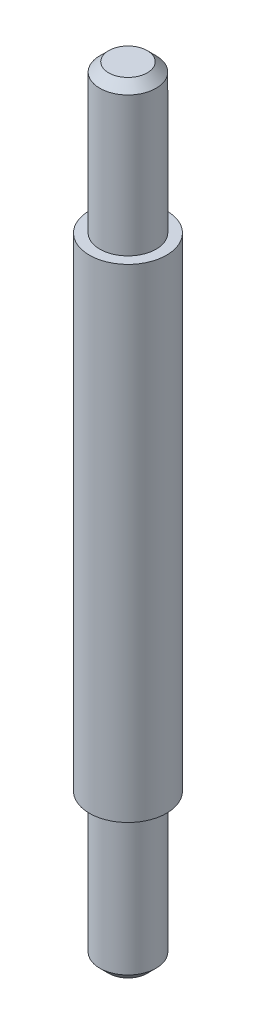
ISO-10303-21;
HEADER;
FILE_DESCRIPTION(('STEP AP214'),'2;1');
FILE_NAME('part.step','',(''),(''),'','','');
FILE_SCHEMA(('AUTOMOTIVE_DESIGN { 1 0 10303 214 1 1 1 1 }'));
ENDSEC;
DATA;
#1=APPLICATION_CONTEXT('core data for automotive mechanical design processes');
#2=APPLICATION_PROTOCOL_DEFINITION('international standard','automotive_design',2000,#1);
#3=PRODUCT_CONTEXT('',#1,'mechanical');
#4=PRODUCT('Part','Part','',(#3));
#5=PRODUCT_RELATED_PRODUCT_CATEGORY('part','',(#4));
#6=PRODUCT_DEFINITION_FORMATION('','',#4);
#7=PRODUCT_DEFINITION_CONTEXT('part definition',#1,'design');
#8=PRODUCT_DEFINITION('design','',#6,#7);
#9=PRODUCT_DEFINITION_SHAPE('','',#8);
#10=(LENGTH_UNIT() NAMED_UNIT(*) SI_UNIT(.MILLI.,.METRE.));
#11=(NAMED_UNIT(*) PLANE_ANGLE_UNIT() SI_UNIT($,.RADIAN.));
#12=(NAMED_UNIT(*) SI_UNIT($,.STERADIAN.) SOLID_ANGLE_UNIT());
#13=UNCERTAINTY_MEASURE_WITH_UNIT(LENGTH_MEASURE(1.E-05),#10,'distance_accuracy_value','');
#14=(GEOMETRIC_REPRESENTATION_CONTEXT(3) GLOBAL_UNCERTAINTY_ASSIGNED_CONTEXT((#13)) GLOBAL_UNIT_ASSIGNED_CONTEXT((#10,
#11,#12)) REPRESENTATION_CONTEXT('',''));
#15=CARTESIAN_POINT('',(0.,0.,0.));
#16=DIRECTION('',(0.,0.,1.));
#17=DIRECTION('',(1.,0.,0.));
#18=AXIS2_PLACEMENT_3D('',#15,#16,#17);
#19=CARTESIAN_POINT('',(0.,131.5,0.));
#20=DIRECTION('',(0.,-1.,0.));
#21=DIRECTION('',(0.,0.,-1.));
#22=AXIS2_PLACEMENT_3D('',#19,#20,#21);
#23=PLANE('',#22);
#24=CARTESIAN_POINT('',(0.,131.5,0.));
#25=DIRECTION('',(0.,-1.,0.));
#26=DIRECTION('',(0.,0.,-1.));
#27=AXIS2_PLACEMENT_3D('',#24,#25,#26);
#28=CIRCLE('',#27,6.50000000000003);
#29=CARTESIAN_POINT('',(0.,131.5,-6.50000000000003));
#30=VERTEX_POINT('',#29);
#31=EDGE_CURVE('E50',#30,#30,#28,.F.);
#32=ORIENTED_EDGE('',*,*,#31,.T.);
#33=EDGE_LOOP('',(#32));
#34=FACE_BOUND('',#33,.T.);
#35=ADVANCED_FACE('F39',(#34),#23,.F.);
#36=CARTESIAN_POINT('',(0.,65.5594059405942,0.));
#37=DIRECTION('',(0.,1.,0.));
#38=DIRECTION('',(0.,0.,1.));
#39=AXIS2_PLACEMENT_3D('',#36,#37,#38);
#40=CYLINDRICAL_SURFACE('',#39,9.49999999999999);
#41=CARTESIAN_POINT('',(0.,128.5,0.));
#42=DIRECTION('',(0.,-1.,0.));
#43=DIRECTION('',(0.,0.,-1.));
#44=AXIS2_PLACEMENT_3D('',#41,#42,#43);
#45=CIRCLE('',#44,9.49999999999999);
#46=CARTESIAN_POINT('',(0.,128.5,-9.49999999999999));
#47=VERTEX_POINT('',#46);
#48=EDGE_CURVE('E10',#47,#47,#45,.T.);
#49=ORIENTED_EDGE('',*,*,#48,.T.);
#50=EDGE_LOOP('',(#49));
#51=FACE_BOUND('',#50,.T.);
#52=CARTESIAN_POINT('',(0.,81.5,0.));
#53=DIRECTION('',(0.,1.,0.));
#54=DIRECTION('',(0.,0.,1.));
#55=AXIS2_PLACEMENT_3D('',#52,#53,#54);
#56=CIRCLE('',#55,9.49999999999999);
#57=CARTESIAN_POINT('',(0.,81.5,9.49999999999999));
#58=VERTEX_POINT('',#57);
#59=EDGE_CURVE('E58',#58,#58,#56,.T.);
#60=ORIENTED_EDGE('',*,*,#59,.T.);
#61=EDGE_LOOP('',(#60));
#62=FACE_BOUND('',#61,.T.);
#63=ADVANCED_FACE('F95',(#51,#62),#40,.T.);
#64=CARTESIAN_POINT('',(9.49999999999999,81.5,0.));
#65=DIRECTION('',(0.,-1.,0.));
#66=DIRECTION('',(0.,0.,-1.));
#67=AXIS2_PLACEMENT_3D('',#64,#65,#66);
#68=PLANE('',#67);
#69=ORIENTED_EDGE('',*,*,#59,.F.);
#70=EDGE_LOOP('',(#69));
#71=FACE_BOUND('',#70,.T.);
#72=CARTESIAN_POINT('',(0.,81.5,0.));
#73=DIRECTION('',(0.,1.,0.));
#74=DIRECTION('',(0.,0.,1.));
#75=AXIS2_PLACEMENT_3D('',#72,#73,#74);
#76=CIRCLE('',#75,13.);
#77=CARTESIAN_POINT('',(0.,81.5,13.));
#78=VERTEX_POINT('',#77);
#79=EDGE_CURVE('E64',#78,#78,#76,.T.);
#80=ORIENTED_EDGE('',*,*,#79,.T.);
#81=EDGE_LOOP('',(#80));
#82=FACE_BOUND('',#81,.T.);
#83=ADVANCED_FACE('F96',(#71,#82),#68,.F.);
#84=CARTESIAN_POINT('',(0.,65.5594059405942,0.));
#85=DIRECTION('',(0.,1.,0.));
#86=DIRECTION('',(0.,0.,1.));
#87=AXIS2_PLACEMENT_3D('',#84,#85,#86);
#88=CYLINDRICAL_SURFACE('',#87,13.);
#89=ORIENTED_EDGE('',*,*,#79,.F.);
#90=EDGE_LOOP('',(#89));
#91=FACE_BOUND('',#90,.T.);
#92=CARTESIAN_POINT('',(0.,-81.5,0.));
#93=DIRECTION('',(0.,1.,0.));
#94=DIRECTION('',(0.,0.,1.));
#95=AXIS2_PLACEMENT_3D('',#92,#93,#94);
#96=CIRCLE('',#95,13.0000000000001);
#97=CARTESIAN_POINT('',(0.,-81.5,13.0000000000001));
#98=VERTEX_POINT('',#97);
#99=EDGE_CURVE('E67',#98,#98,#96,.T.);
#100=ORIENTED_EDGE('',*,*,#99,.T.);
#101=EDGE_LOOP('',(#100));
#102=FACE_BOUND('',#101,.T.);
#103=ADVANCED_FACE('F86',(#91,#102),#88,.T.);
#104=CARTESIAN_POINT('',(13.0000000000001,-81.5,0.));
#105=DIRECTION('',(0.,1.,0.));
#106=DIRECTION('',(0.,0.,1.));
#107=AXIS2_PLACEMENT_3D('',#104,#105,#106);
#108=PLANE('',#107);
#109=ORIENTED_EDGE('',*,*,#99,.F.);
#110=EDGE_LOOP('',(#109));
#111=FACE_BOUND('',#110,.T.);
#112=CARTESIAN_POINT('',(0.,-81.5,0.));
#113=DIRECTION('',(0.,1.,0.));
#114=DIRECTION('',(0.,0.,1.));
#115=AXIS2_PLACEMENT_3D('',#112,#113,#114);
#116=CIRCLE('',#115,9.5);
#117=CARTESIAN_POINT('',(0.,-81.5,9.5));
#118=VERTEX_POINT('',#117);
#119=EDGE_CURVE('E69',#118,#118,#116,.T.);
#120=ORIENTED_EDGE('',*,*,#119,.T.);
#121=EDGE_LOOP('',(#120));
#122=FACE_BOUND('',#121,.T.);
#123=ADVANCED_FACE('F71',(#111,#122),#108,.F.);
#124=CARTESIAN_POINT('',(0.,65.5594059405942,0.));
#125=DIRECTION('',(0.,1.,0.));
#126=DIRECTION('',(0.,0.,1.));
#127=AXIS2_PLACEMENT_3D('',#124,#125,#126);
#128=CYLINDRICAL_SURFACE('',#127,9.50000000000001);
#129=CARTESIAN_POINT('',(0.,-128.5,0.));
#130=DIRECTION('',(0.,1.,0.));
#131=DIRECTION('',(0.,0.,1.));
#132=AXIS2_PLACEMENT_3D('',#129,#130,#131);
#133=CIRCLE('',#132,9.50000000000001);
#134=CARTESIAN_POINT('',(0.,-128.5,9.5));
#135=VERTEX_POINT('',#134);
#136=EDGE_CURVE('E54',#135,#135,#133,.T.);
#137=ORIENTED_EDGE('',*,*,#136,.T.);
#138=EDGE_LOOP('',(#137));
#139=FACE_BOUND('',#138,.T.);
#140=ORIENTED_EDGE('',*,*,#119,.F.);
#141=EDGE_LOOP('',(#140));
#142=FACE_BOUND('',#141,.T.);
#143=ADVANCED_FACE('F73',(#139,#142),#128,.T.);
#144=CARTESIAN_POINT('',(9.50000000000002,-131.5,0.));
#145=DIRECTION('',(0.,1.,0.));
#146=DIRECTION('',(0.,0.,1.));
#147=AXIS2_PLACEMENT_3D('',#144,#145,#146);
#148=PLANE('',#147);
#149=CARTESIAN_POINT('',(0.,-131.5,0.));
#150=DIRECTION('',(0.,1.,0.));
#151=DIRECTION('',(0.,0.,1.));
#152=AXIS2_PLACEMENT_3D('',#149,#150,#151);
#153=CIRCLE('',#152,6.50000000000003);
#154=CARTESIAN_POINT('',(0.,-131.5,6.50000000000002));
#155=VERTEX_POINT('',#154);
#156=EDGE_CURVE('E51',#155,#155,#153,.F.);
#157=ORIENTED_EDGE('',*,*,#156,.T.);
#158=EDGE_LOOP('',(#157));
#159=FACE_BOUND('',#158,.T.);
#160=ADVANCED_FACE('F80',(#159),#148,.F.);
#161=CARTESIAN_POINT('',(0.,-128.5,0.));
#162=DIRECTION('',(0.,1.,0.));
#163=DIRECTION('',(0.,0.,1.));
#164=AXIS2_PLACEMENT_3D('',#161,#162,#163);
#165=CONICAL_SURFACE('',#164,9.50000000000001,0.785398163397449);
#166=CARTESIAN_POINT('',(0.,-131.5,6.50000000000002));
#167=CARTESIAN_POINT('',(0.,-131.46875,6.53125000000002));
#168=CARTESIAN_POINT('',(0.,-131.4375,6.56250000000002));
#169=CARTESIAN_POINT('',(0.,-131.375,6.62500000000002));
#170=CARTESIAN_POINT('',(0.,-131.34375,6.65625000000002));
#171=CARTESIAN_POINT('',(0.,-131.28125,6.71875000000002));
#172=CARTESIAN_POINT('',(0.,-131.25,6.75000000000002));
#173=CARTESIAN_POINT('',(0.,-131.1875,6.81250000000002));
#174=CARTESIAN_POINT('',(0.,-131.15625,6.84375000000002));
#175=CARTESIAN_POINT('',(0.,-131.09375,6.90625000000002));
#176=CARTESIAN_POINT('',(0.,-131.0625,6.93750000000002));
#177=CARTESIAN_POINT('',(0.,-131.,7.00000000000001));
#178=CARTESIAN_POINT('',(0.,-130.96875,7.03125000000001));
#179=CARTESIAN_POINT('',(0.,-130.90625,7.09375000000001));
#180=CARTESIAN_POINT('',(0.,-130.875,7.12500000000002));
#181=CARTESIAN_POINT('',(0.,-130.8125,7.18750000000002));
#182=CARTESIAN_POINT('',(0.,-130.78125,7.21875000000001));
#183=CARTESIAN_POINT('',(0.,-130.71875,7.28125000000001));
#184=CARTESIAN_POINT('',(0.,-130.6875,7.31250000000001));
#185=CARTESIAN_POINT('',(0.,-130.625,7.37500000000001));
#186=CARTESIAN_POINT('',(0.,-130.59375,7.40625000000001));
#187=CARTESIAN_POINT('',(0.,-130.53125,7.46875000000001));
#188=CARTESIAN_POINT('',(0.,-130.5,7.50000000000001));
#189=CARTESIAN_POINT('',(0.,-130.4375,7.56250000000001));
#190=CARTESIAN_POINT('',(0.,-130.40625,7.59375000000001));
#191=CARTESIAN_POINT('',(0.,-130.34375,7.65625000000001));
#192=CARTESIAN_POINT('',(0.,-130.3125,7.68750000000001));
#193=CARTESIAN_POINT('',(0.,-130.25,7.75000000000001));
#194=CARTESIAN_POINT('',(0.,-130.21875,7.78125000000001));
#195=CARTESIAN_POINT('',(0.,-130.15625,7.84375000000001));
#196=CARTESIAN_POINT('',(0.,-130.125,7.87500000000001));
#197=CARTESIAN_POINT('',(0.,-130.0625,7.93750000000001));
#198=CARTESIAN_POINT('',(0.,-130.03125,7.96875000000001));
#199=CARTESIAN_POINT('',(0.,-129.96875,8.03125000000001));
#200=CARTESIAN_POINT('',(0.,-129.9375,8.06250000000001));
#201=CARTESIAN_POINT('',(0.,-129.875,8.12500000000001));
#202=CARTESIAN_POINT('',(0.,-129.84375,8.15625000000001));
#203=CARTESIAN_POINT('',(0.,-129.78125,8.21875000000001));
#204=CARTESIAN_POINT('',(0.,-129.75,8.25));
#205=CARTESIAN_POINT('',(0.,-129.6875,8.3125));
#206=CARTESIAN_POINT('',(0.,-129.65625,8.34375000000001));
#207=CARTESIAN_POINT('',(0.,-129.59375,8.40625000000001));
#208=CARTESIAN_POINT('',(0.,-129.5625,8.43750000000001));
#209=CARTESIAN_POINT('',(0.,-129.5,8.5));
#210=CARTESIAN_POINT('',(0.,-129.46875,8.53125));
#211=CARTESIAN_POINT('',(0.,-129.40625,8.59375));
#212=CARTESIAN_POINT('',(0.,-129.375,8.625));
#213=CARTESIAN_POINT('',(0.,-129.3125,8.6875));
#214=CARTESIAN_POINT('',(0.,-129.28125,8.71875));
#215=CARTESIAN_POINT('',(0.,-129.21875,8.78125));
#216=CARTESIAN_POINT('',(0.,-129.1875,8.8125));
#217=CARTESIAN_POINT('',(0.,-129.125,8.875));
#218=CARTESIAN_POINT('',(0.,-129.09375,8.90625));
#219=CARTESIAN_POINT('',(0.,-129.03125,8.96875000000001));
#220=CARTESIAN_POINT('',(0.,-129.,9.));
#221=CARTESIAN_POINT('',(0.,-128.9375,9.0625));
#222=CARTESIAN_POINT('',(0.,-128.90625,9.09375));
#223=CARTESIAN_POINT('',(0.,-128.84375,9.15625));
#224=CARTESIAN_POINT('',(0.,-128.8125,9.1875));
#225=CARTESIAN_POINT('',(0.,-128.75,9.25));
#226=CARTESIAN_POINT('',(0.,-128.71875,9.28125));
#227=CARTESIAN_POINT('',(0.,-128.65625,9.34375));
#228=CARTESIAN_POINT('',(0.,-128.625,9.375));
#229=CARTESIAN_POINT('',(0.,-128.5625,9.4375));
#230=CARTESIAN_POINT('',(0.,-128.53125,9.46875));
#231=CARTESIAN_POINT('',(0.,-128.5,9.5));
#232=B_SPLINE_CURVE_WITH_KNOTS('',3,(#166,#167,#168,#169,#170,#171,#172,#173,#174,#175,#176,
#177,#178,#179,#180,#181,#182,#183,#184,#185,#186,#187,#188,#189,#190,#191,#192,#193,#194,#195,
#196,#197,#198,#199,#200,#201,#202,#203,#204,#205,#206,#207,#208,#209,#210,#211,#212,#213,#214,
#215,#216,#217,#218,#219,#220,#221,#222,#223,#224,#225,#226,#227,#228,#229,#230,#231),
.UNSPECIFIED.,.F.,.F.,(4,2,2,2,2,2,2,2,2,2,2,2,2,2,2,2,2,2,2,2,2,2,2,2,2,2,2,2,2,2,2,2,4),(0.,
0.13258252147248,0.265165042944959,0.397747564417439,0.530330085889919,0.662912607362399,
0.795495128834879,0.928077650307338,1.06066017177982,1.1932426932523,1.32582521472478,
1.45840773619726,1.59099025766974,1.7235727791422,1.85615530061468,1.98873782208716,
2.12132034355964,2.25390286503212,2.3864853865046,2.51906790797708,2.65165042944954,
2.78423295092201,2.91681547239449,3.04939799386697,3.18198051533945,3.31456303681193,
3.44714555828439,3.57972807975687,3.71231060122935,3.84489312270183,3.97747564417431,
4.11005816564679,4.24264068711927),.UNSPECIFIED.);
#233=EDGE_CURVE('BSEAM84',#155,#135,#232,.T.);
#234=ORIENTED_EDGE('',*,*,#156,.F.);
#235=ORIENTED_EDGE('',*,*,#136,.F.);
#236=ORIENTED_EDGE('',*,*,#233,.T.);
#237=ORIENTED_EDGE('',*,*,#233,.F.);
#238=EDGE_LOOP('',(#234,#236,#235,#237));
#239=FACE_BOUND('',#238,.T.);
#240=ADVANCED_FACE('F84',(#239),#165,.T.);
#241=CARTESIAN_POINT('',(0.,131.5,0.));
#242=DIRECTION('',(0.,-1.,0.));
#243=DIRECTION('',(0.,0.,-1.));
#244=AXIS2_PLACEMENT_3D('',#241,#242,#243);
#245=CONICAL_SURFACE('',#244,6.50000000000003,0.785398163397441);
#246=ORIENTED_EDGE('',*,*,#48,.F.);
#247=EDGE_LOOP('',(#246));
#248=FACE_BOUND('',#247,.T.);
#249=ORIENTED_EDGE('',*,*,#31,.F.);
#250=EDGE_LOOP('',(#249));
#251=FACE_BOUND('',#250,.T.);
#252=ADVANCED_FACE('F45',(#248,#251),#245,.T.);
#253=CLOSED_SHELL('',(#35,#63,#83,#103,#123,#143,#160,#240,#252));
#254=MANIFOLD_SOLID_BREP('B2',#253);
#255=ADVANCED_BREP_SHAPE_REPRESENTATION('',(#18,#254),#14);
#256=SHAPE_DEFINITION_REPRESENTATION(#9,#255);
ENDSEC;
END-ISO-10303-21;
